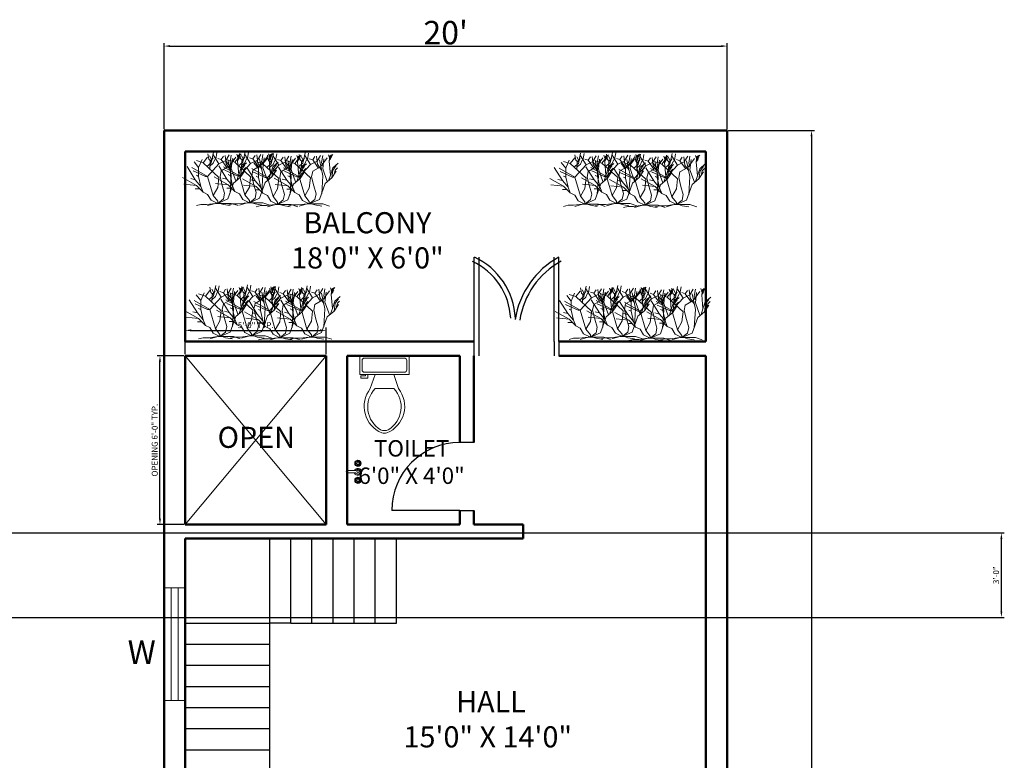
# Model space of a CAD drawing. Units: inches. Extents: x 995 to 2141, y 2161 to 2928.
# Tile 7 of 7: x 1721 to 2141, y 2613 to 2928. Entities that reach past the tile are written whole.
import ezdxf

# ---------------------------------------------------------------- set-up
doc = ezdxf.new("R2010")
doc.units = ezdxf.units.IN
for name, color, linetype, lineweight in [('A-ANNO-DIMS', 2, 'Continuous', 18), ('A-ANNO-TEXT', 7, 'Continuous', 18), ('A-AREA-IDEN', 7, 'Continuous', 25), ('A-DOOR', 3, 'Continuous', 25), ('A-FLOR-FIXT', 9, 'Continuous', 18), ('A-FLOR-OPEN', 8, 'Continuous', 13), ('A-FLOR-STRS', 7, 'Continuous', 25), ('A-GLAZ', 4, 'Continuous', 18), ('A-WALL', 7, 'Continuous', 50), ('L-PLNT-TREE', 94, 'Continuous', 13)]:
    doc.layers.add(name, color=color, linetype=linetype, lineweight=lineweight)
doc.styles.get("Standard").update_dxf_attribs({"font": 'arial.ttf'})
doc.dimstyles.new('ISO-25', dxfattribs={"dimtxt": 2.5, "dimasz": 2.5, "dimexe": 1.25, "dimexo": 0.625, "dimtad": 1, "dimdec": 0, "dimlunit": 3, "dimtxsty": 'Standard', "dimcen": 2.5, "dimadec": 0, "dimazin": 0, "dimtfac": 1, "dimtdec": 0, "dimtmove": 0, "dimatfit": 3, "dimfxl": 1, "dimarcsym": 0})

# ---------------------------------------------------------------- blocks, each defined once
blk = doc.blocks.new('*U15')
for p, q in [((-12.471, 19.775), (-12.898, 22.044)), ((-11.28, 19.619), (-12.104, 21.184)), ((-11.433, 18.289), (-10.457, 22.749)), ((-8.16, 17.76), (-10.56, 21.6)), ((-9.48, 19.775), (-8.992, 22.592)), ((-7.2, 19.68), (-6.24, 21.12)), ((-5.086, 17.741), (-5.513, 21.34)), ((-5.28, 19.2), (-3.84, 21.6)), ((-3.377, 18.602), (-2.888, 21.575)), ((-0.508, 21.888), (-0.081, 20.558)), ((-0.203, 19.149), (0.102, 21.34)), ((-0.02, 20.01), (0.896, 21.105)), ((0.041, 20.714), (1.384, 22.044)), ((0.102, 21.34), (0.835, 21.888)), ((-16.8, 16.32), (-18.72, 18.72)), ((-14.88, 18.24), (-17.76, 19.2)), ((-16.8, 16.32), (-15.36, 19.68)), ((-14.88, 18.24), (-12.96, 20.64)), ((-8.16, 12), (-14.88, 18.24)), ((-13.325, 16.724), (-11.433, 18.289)), ((-12.96, 12.48), (-8.16, 17.76)), ((-11.677, 19.071), (-12.471, 19.775)), ((-12.043, 15.628), (-11.921, 18.836)), ((-11.982, 16.802), (-10.579, 18.054)), ((-11.921, 18.836), (-10.64, 20.401)), ((-10.579, 18.054), (-9.846, 19.697)), ((-7.2, 19.68), (-8.64, 20.16)), ((-8.16, 17.76), (-5.28, 19.2)), ((-4.8, 16.32), (-7.2, 19.68)), ((-7.2, 14.88), (-3.84, 16.8)), ((-3.377, 15.315), (-5.086, 17.819)), ((-2.88, 12.96), (-4.32, 19.68)), ((-3.84, 16.8), (-0.96, 20.64)), ((-2.766, 16.802), (-3.377, 18.602)), ((-2.88, 15.84), (-2.4, 20.16)), ((0.346, 13.203), (-0.203, 19.149)), ((-0.142, 19.384), (0.59, 20.401)), ((1.323, 16.254), (3.642, 18.289)), ((1.44, 15.36), (2.88, 17.28)), ((-18.24, 11.04), (-21.755, 16.655)), ((-12.96, 12.48), (-19.68, 16.32)), ((-13.92, 12.48), (-19.2, 14.88)), ((-16.8, 12.48), (-17.76, 12.96)), ((-16.8, 12.48), (-16.8, 16.32)), ((-7.68, 12.48), (-7.2, 14.88)), ((-3.36, 5.28), (-2.88, 12.96)), ((-0.96, 10.56), (-2.88, 15.84)), ((-0.48, 10.8), (0.346, 13.203)), ((0.346, 13.203), (1.323, 16.254)), ((0.96, 12), (1.44, 15.36)), ((0.96, 12), (2.88, 14.88)), ((1.92, 13.44), (2.4, 15.36)), ((2.4, 15.36), (3.36, 16.32)), ((-17.76, 8.64), (-23.663, 11.961)), ((-17.76, 8.64), (-23.128, 9.222)), ((-18.24, 11.04), (-20.16, 11.52)), ((-15.84, 8.16), (-18.24, 11.04)), ((-14.88, 5.76), (-17.76, 8.64)), ((-15.84, 8.16), (-16.8, 12.48)), ((-12.96, 12.48), (-13.92, 12.48)), ((-10.56, 4.32), (-12.96, 12.48)), ((-8.64, 7.68), (-8.16, 12)), ((-6.72, 8.64), (-7.68, 12.48)), ((-5.76, 5.28), (-6.72, 8.64)), ((-4.32, 2.88), (-1.92, 9.6)), ((-1.92, 9.6), (0.96, 12)), ((-16.32, 7.2), (-18.24, 7.2)), ((-14.88, 5.76), (-15.84, 8.16)), ((-12.96, 4.8), (-14.88, 5.76)), ((-11.52, 2.4), (-12.96, 4.8)), ((-10.56, 4.32), (-8.64, 7.68)), ((-8.64, 1.92), (-10.56, 4.32)), ((-6.24, 2.88), (-5.76, 5.28)), ((-15.84, 0.48), (-17.76, 0)), ((-13.44, 0.48), (-15.84, 0.48)), ((-9.6, 0.96), (-13.44, 0.48)), ((-9.6, 0.96), (-12.96, 0)), ((-8.64, 0.96), (-11.52, 2.4)), ((-9.6, 0.96), (-7.68, 0.96)), ((-8.64, 0.96), (-4.32, 2.88)), ((-8.64, 0.96), (-6.24, 2.88)), ((-8.64, 0.96), (-8.64, 1.92)), ((-8.64, 0.96), (-2.88, 0.96)), ((-7.68, 0.96), (-6.24, 0.48)), ((-6.24, 0.48), (-3.36, 0)), ((-2.88, 0.96), (0, 0))]:
    blk.add_line(p, q)
blk = doc.blocks.new('Toilet - top')
for p, q in [((9.5, -6), (9.5, -2)), ((-8, -8.5), (-8, -8)), ((-7, -8), (-7, -9.5)), ((-4, -8), (-6, -14)), ((4, -8), (6, -14)), ((-10, -8.5), (-8, -8.5)), ((-10, -9.5), (-10, -8.5)), ((-7, -9.5), (-10, -9.5)), ((4, -14), (-4, -14))]:
    blk.add_line(p, q)
blk.add_lwpolyline([(10.5, -8), (10.5, 0), (-10.5, 0), (-10.5, -8)], close=True)
for points in [[(-9.5, -2), (-9.5, -6)], [(8.5, -1), (-8.5, -1)], [(-8.5, -7), (8.5, -7)]]:
    blk.add_lwpolyline(points)
for centre, radius, start, end in [((-8.62, -1.88), 0.884, 81.8699, 188.1301), ((8.62, -1.88), 0.884, 351.8699, 98.1301), ((-8.62, -6.12), 0.884, 171.8699, 278.1301), ((8.62, -6.12), 0.884, 261.8699, 8.1301), ((3.52, -21.58), 12.17, 141.4691, 247.9714), ((4.2, -21.82), 11.33, 136.3677, 238.9468), ((-3.52, -21.58), 12.17, 292.0284, 38.5307), ((-4.2, -21.82), 11.33, 301.053, 43.6321), ((0, -27.88), 4, 245.7318, 294.2682), ((0, -29), 4, 254.8605, 285.1395)]:
    blk.add_arc(centre, radius, start, end)
blk = doc.blocks.new('Faucet - Bathroom top')
for p, q in [((-4.107, 0.125), (-4.375, 0.125)), ((-3.75, 0.4788), (-3.75, 0.75)), ((-3.5, 0.482), (-3.5, 0.75)), ((-3.1461, 0.125), (-2.875, 0.125)), ((3.143, 0.125), (2.875, 0.125)), ((3.5, 0.4788), (3.5, 0.75)), ((3.75, 0.482), (3.75, 0.75)), ((4.1039, 0.125), (4.375, 0.125)), ((-4.1039, -0.125), (-4.375, -0.125)), ((-3.75, -0.4821), (-3.75, -0.75)), ((-3.5, -0.4789), (-3.5, -0.75)), ((-3.143, -0.125), (-2.875, -0.125)), ((-0.5, -0.8639), (-0.5, -4.5)), ((0.5, -4.5), (0.5, -0.8631)), ((3.1461, -0.125), (2.875, -0.125)), ((3.5, -0.4821), (3.5, -0.75)), ((3.75, -0.4789), (3.75, -0.75)), ((4.107, -0.125), (4.375, -0.125))]:
    blk.add_line(p, q)
for centre, radius in [((-3.625, 0), 1.375), ((-4.625, 0), 0.2795), ((-3.625, 0), 0.5), ((-3.625, 1), 0.2795), ((-2.625, 0), 0.2795), ((0, 0), 0.5), ((3.625, 0), 1.375), ((2.625, 0), 0.2795), ((3.625, 0), 0.5), ((3.625, 1), 0.2795), ((4.625, 0), 0.2795), ((-3.625, -1), 0.2795), ((3.625, -1), 0.2795)]:
    blk.add_circle(centre, radius)
for centre, radius, start, end in [((-3.625, 0), 1, 105.2407, 164.2093), ((-3.625, 0), 1, 16.44125, 74.07887), ((0, 0), 1.5, 289.6514, 250.3603), ((0, 0), 1, 300.3431, 239.7554), ((3.625, 0), 1, 106.12, 164.0884), ((3.625, 0), 1, 16.23422, 73.90469), ((-3.625, 0), 1, 196.2342, 253.9047), ((-3.625, 0), 1, 286.12, 344.0884), ((3.625, 0), 1, 196.4413, 254.0789), ((3.625, 0), 1, 285.2407, 344.2093), ((0, -4.5), 0.5, 180, 0)]:
    blk.add_arc(centre, radius, start, end)
blk = doc.blocks.new('*D19')
at = {"layer": 'A-ANNO-DIMS', "color": 0, "lineweight": -2, "transparency": 16777216}
for p, q in [((1783.1, 2881.73), (1783.1, 2918.35)), ((2023.1, 2881.73), (2023.1, 2918.35)), ((1785.6, 2917.1), (2020.6, 2917.1))]:
    blk.add_line(p, q, dxfattribs=at)
at = {"layer": 'A-ANNO-DIMS', "color": 0, "transparency": 16777216}
for points in [[(1785.6, 2917.52), (1785.6, 2916.68), (1783.1, 2917.1)], [(2020.6, 2917.52), (2020.6, 2916.68), (2023.1, 2917.1)]]:
    blk.add_solid(points, dxfattribs=at)
at = {"layer": 'Defpoints', "color": 0, "transparency": 16777216}
for p in [(2023.1, 2917.1), (1783.1, 2881.1), (2023.1, 2881.1)]:
    blk.add_point(p, dxfattribs=at)
at = {"layer": 'A-ANNO-DIMS', "color": 0, "transparency": 16777216, "insert": (1903.1, 2922.83), "char_height": 2.5, "attachment_point": 5}
blk.add_mtext("{\\H4x;20'}", dxfattribs=at)
blk = doc.blocks.new('*D20')
at = {"layer": 'A-ANNO-DIMS', "color": 0, "lineweight": -2, "transparency": 16777216}
for p, q in [((2023.72, 2881.1), (2060.35, 2881.1)), ((2059.1, 2878.6), (2059.1, 2283.6)), ((2023.72, 2281.1), (2060.35, 2281.1))]:
    blk.add_line(p, q, dxfattribs=at)
at = {"layer": 'A-ANNO-DIMS', "color": 0, "transparency": 16777216}
for points in [[(2058.68, 2878.6), (2059.51, 2878.6), (2059.1, 2881.1)], [(2058.68, 2283.6), (2059.51, 2283.6), (2059.1, 2281.1)]]:
    blk.add_solid(points, dxfattribs=at)
at = {"layer": 'Defpoints', "color": 0, "transparency": 16777216}
for p in [(2023.1, 2881.1), (2023.1, 2281.1), (2059.1, 2281.1)]:
    blk.add_point(p, dxfattribs=at)
at = {"layer": 'A-ANNO-DIMS', "color": 0, "transparency": 16777216, "insert": (2053.37, 2581.1), "char_height": 2.5, "attachment_point": 5, "rotation": 90}
blk.add_mtext("{\\H4x;50'}", dxfattribs=at)
blk = doc.blocks.new('WIN-48IN')
for p, q in [((0, 48), (0, 0)), ((9, 48), (0, 48)), ((3, 48), (3, 0)), ((6, 0), (6, 48)), ((9, 0), (9, 48)), ((0, 0), (9, 0))]:
    blk.add_line(p, q)
blk = doc.blocks.new('OPENING-CROSS-60X72')
for p, q in [((60, 72), (0, 0)), ((0, 72), (60, 0))]:
    blk.add_line(p, q)
blk = doc.blocks.new('*D38')
at = {"layer": 'A-ANNO-DIMS', "color": 0, "lineweight": -2, "transparency": 16777216}
for p, q in [((1791.47, 2785.1), (1780.05, 2785.1)), ((1781.3, 2715.6), (1781.3, 2782.6)), ((1791.47, 2713.1), (1780.05, 2713.1))]:
    blk.add_line(p, q, dxfattribs=at)
at = {"layer": 'A-ANNO-DIMS', "color": 0, "transparency": 16777216}
for points in [[(1780.88, 2782.6), (1781.71, 2782.6), (1781.3, 2785.1)], [(1780.88, 2715.6), (1781.71, 2715.6), (1781.3, 2713.1)]]:
    blk.add_solid(points, dxfattribs=at)
at = {"layer": 'Defpoints', "color": 0, "transparency": 16777216}
for p in [(1781.3, 2785.1), (1792.1, 2785.1), (1792.1, 2713.1)]:
    blk.add_point(p, dxfattribs=at)
at = {"layer": 'A-ANNO-DIMS', "color": 0, "transparency": 16777216, "insert": (1779.38, 2749.1), "char_height": 2.5, "attachment_point": 5, "rotation": 90}
blk.add_mtext('OPENING 6\'-0" TYP.', dxfattribs=at)
blk = doc.blocks.new('*D39')
at = {"layer": 'A-ANNO-DIMS', "color": 0, "lineweight": -2, "transparency": 16777216}
for p, q in [((1792.1, 2785.73), (1792.1, 2797.15)), ((1852.1, 2785.73), (1852.1, 2797.15)), ((1794.6, 2795.9), (1849.6, 2795.9))]:
    blk.add_line(p, q, dxfattribs=at)
at = {"layer": 'A-ANNO-DIMS', "color": 0, "transparency": 16777216}
for points in [[(1794.6, 2796.32), (1794.6, 2795.48), (1792.1, 2795.9)], [(1849.6, 2796.32), (1849.6, 2795.48), (1852.1, 2795.9)]]:
    blk.add_solid(points, dxfattribs=at)
at = {"layer": 'Defpoints', "color": 0, "transparency": 16777216}
for p in [(1852.1, 2795.9), (1792.1, 2785.1), (1852.1, 2785.1)]:
    blk.add_point(p, dxfattribs=at)
at = {"layer": 'A-ANNO-DIMS', "color": 0, "transparency": 16777216, "insert": (1822.1, 2797.8), "char_height": 2.5, "attachment_point": 5}
blk.add_mtext('5\'-0" TYP.', dxfattribs=at)
blk = doc.blocks.new('*D64')
at = {"layer": 'A-ANNO-DIMS', "color": 0, "lineweight": -2, "transparency": 16777216}
for p, q in [((1532.63, 2709.52), (2141.3, 2709.52)), ((2140.05, 2676.02), (2140.05, 2707.02)), ((1532.63, 2673.52), (2141.3, 2673.52))]:
    blk.add_line(p, q, dxfattribs=at)
at = {"layer": 'A-ANNO-DIMS', "color": 0, "transparency": 16777216}
for points in [[(2139.63, 2707.02), (2140.46, 2707.02), (2140.05, 2709.52)], [(2139.63, 2676.02), (2140.46, 2676.02), (2140.05, 2673.52)]]:
    blk.add_solid(points, dxfattribs=at)
at = {"layer": 'Defpoints', "color": 0, "transparency": 16777216}
for p in [(1532, 2709.52), (2140.05, 2709.52), (1532, 2673.52)]:
    blk.add_point(p, dxfattribs=at)
at = {"layer": 'A-ANNO-DIMS', "color": 0, "transparency": 16777216, "insert": (2138.14, 2691.52), "char_height": 2.5, "attachment_point": 5, "rotation": 90}
blk.add_mtext('3\'-0"', dxfattribs=at)

msp = doc.modelspace()

# ---------------------------------------------------------------- linework, layer by layer
at = {"layer": 'A-DOOR'}
for p, q in [((1915.33, 2791.1), (1915.33, 2827.1)), ((1917.33, 2791.1), (1917.33, 2827.1)), ((1949.33, 2791.1), (1949.33, 2827.1)), ((1951.33, 2791.1), (1951.33, 2827.1)), ((1915.33, 2785.1), (1915.33, 2791.1)), ((1917.33, 2785.1), (1917.33, 2791.1)), ((1949.33, 2791.1), (1949.33, 2785.1)), ((1951.33, 2791.1), (1951.33, 2785.1)), ((1915.1, 2748.1), (1909.1, 2748.1)), ((1909.1, 2719.1), (1880.1, 2719.1)), ((1909.1, 2719.1), (1915.1, 2719.1))]:
    msp.add_line(p, q, dxfattribs=at)
for centre, radius, start, end in [((1902.65, 2799.67), 30.22, 2.781, 65.1814), ((1969.03, 2794.92), 36.73, 118.8094, 171.2426), ((1969.03, 2794.92), 34.73, 118.8094, 171.2426), ((1902.65, 2799.67), 28.22, 2.781, 65.1814), ((1909.1, 2719.1), 29, 90, 180)]:
    msp.add_arc(centre, radius, start, end, dxfattribs=at)
at = {"layer": 'A-FLOR-STRS'}
for p, q in [((1828.1, 2539.1), (1828.1, 2707.1)), ((1837.1, 2671.1), (1837.1, 2707.1)), ((1846.1, 2671.1), (1846.1, 2707.1)), ((1855.1, 2671.1), (1855.1, 2707.1)), ((1864.1, 2671.1), (1864.1, 2707.1)), ((1873.1, 2671.1), (1873.1, 2707.1)), ((1882.1, 2671.1), (1882.1, 2707.1)), ((1792.1, 2671.1), (1828.1, 2671.1)), ((1837.1, 2671.1), (1828.1, 2671.1)), ((1837.1, 2671.1), (1882.1, 2671.1)), ((1792.1, 2662.1), (1828.1, 2662.1)), ((1792.1, 2653.1), (1828.1, 2653.1)), ((1792.1, 2644.1), (1828.1, 2644.1)), ((1792.1, 2635.1), (1828.1, 2635.1)), ((1792.1, 2626.1), (1828.1, 2626.1)), ((1792.1, 2617.1), (1828.1, 2617.1))]:
    msp.add_line(p, q, dxfattribs=at)
at = {"layer": 'A-WALL'}
for p, q in [((1783.1, 2881.1), (2023.1, 2881.1)), ((1783.1, 2281.1), (1783.1, 2881.1)), ((2023.1, 2881.1), (2023.1, 2281.1)), ((1792.1, 2872.1), (2014.1, 2872.1)), ((1792.1, 2791.1), (1792.1, 2872.1)), ((2014.1, 2872.1), (2014.1, 2791.1)), ((1792.1, 2791.1), (1915.33, 2791.1)), ((1951.33, 2791.1), (2014.1, 2791.1)), ((1792.1, 2785.1), (1852.1, 2785.1)), ((1792.1, 2713.1), (1792.1, 2785.1)), ((1792.1, 2713.1), (1792.1, 2785.1)), ((1852.1, 2713.1), (1852.1, 2785.1)), ((1861.1, 2785.1), (1909.1, 2785.1)), ((1861.1, 2713.1), (1861.1, 2785.1)), ((1909.1, 2748.1), (1909.1, 2785.1)), ((1915.1, 2785.1), (1915.33, 2785.1)), ((1915.1, 2748.1), (1915.1, 2785.1)), ((1951.33, 2785.1), (2014.1, 2785.1)), ((2014.1, 2785.1), (2014.1, 2713.1)), ((1909.1, 2713.1), (1909.1, 2719.1)), ((1909.1, 2713.1), (1909.1, 2719.1)), ((1915.1, 2713.1), (1915.1, 2719.1)), ((1792.1, 2713.1), (1852.1, 2713.1)), ((1861.1, 2713.1), (1909.1, 2713.1)), ((1915.1, 2713.1), (1936.1, 2713.1)), ((1936.1, 2713.1), (1936.1, 2707.1)), ((2014.1, 2713.1), (2014.1, 2699.43)), ((1792.1, 2707.1), (1936.1, 2707.1)), ((1792.1, 2539.1), (1792.1, 2707.1)), ((2014.1, 2707.1), (2014.1, 2539.1))]:
    msp.add_line(p, q, dxfattribs=at)

# ---------------------------------------------------------------- block references
at = {"layer": 'A-FLOR-FIXT'}
msp.add_blockref('Toilet - top', (1876.99, 2785.06), dxfattribs=at)
at = {"layer": 'A-FLOR-FIXT', "rotation": 270}
msp.add_blockref('Faucet - Bathroom top', (1865.7, 2735.59), dxfattribs=at)
at = {"layer": 'A-FLOR-OPEN'}
msp.add_blockref('OPENING-CROSS-60X72', (1792.1, 2713.1), dxfattribs=at)
at = {"layer": 'A-GLAZ'}
msp.add_blockref('WIN-48IN', (1783.1, 2638.1), dxfattribs=at)
at = {"layer": 'L-PLNT-TREE'}
for p in [(1814.59, 2849.07), (1828.1, 2849.33), (1853.61, 2848.87), (1971.12, 2848.75), (1984.63, 2849.01), (1840.1, 2848.61), (1996.63, 2848.29), (2010.14, 2848.55), (1815.52, 2792.28), (1829.03, 2792.54), (1841.03, 2791.82), (1854.54, 2792.08), (1973.46, 2792.03), (1986.97, 2792.29), (1998.97, 2791.57), (2012.48, 2791.83)]:
    msp.add_blockref('*U15', p, dxfattribs=at)

# ---------------------------------------------------------------- texts
at = {"layer": 'A-ANNO-TEXT', "insert": (1767.52, 2663.71), "char_height": 10, "attachment_point": 1}
msp.add_mtext_dynamic_manual_height_columns('W', width=112.484, gutter_width=12.5, heights=[0], dxfattribs=at)
at = {"layer": 'A-AREA-IDEN', "attachment_point": 1}
for s, width, insert, char_height in [('\\pxqc;BALCONY \\P18\'0" X 6\'0"', 118.2971, (1810.6, 2846.29), 9), ('\\pxqc;OPEN ', 52.2467, (1796.26, 2754.81), 9), ('\\pxqc;TOILET\\P6\'0" X 4\'0"', 53.0246, (1862.07, 2749.1), 7), ('\\pxqc; HALL \\P15\'0" X 14\'0"', 103.3264, (1869.4, 2642.11), 9)]:
    msp.add_mtext_dynamic_manual_height_columns(s, width=width, gutter_width=12.5, heights=[0], dxfattribs=dict(at, insert=insert, char_height=char_height))

# ---------------------------------------------------------------- dimensions: what is measured, and where the dimension line sits
at = {"layer": 'A-ANNO-DIMS'}
for base, p1, p2, text, override, picture, middle in [((2023.1, 2917.1), (1783.1, 2881.1), (2023.1, 2881.1), "{\\H4x;20'}", {"dimclrd": 0, "dimclre": 0, "dimclrt": 0}, '*D19', (1903.1, 2922.83)), ((1852.1, 2795.9), (1792.1, 2785.1), (1852.1, 2785.1), '<> TYP.', {"dimdec": 1, "dimlfac": 1, "dimrnd": 0, "dimzin": 1, "dimdsep": 46, "dimlunit": 4, "dimfrac": 2}, '*D39', (1822.1, 2797.8))]:
    dim = msp.add_linear_dim(base=base, p1=p1, p2=p2, text=text, dimstyle='ISO-25', override=override, dxfattribs=at)
    dim.commit()
    dim.dimension.update_dxf_attribs({"geometry": picture, "text_midpoint": middle})
for base, p1, p2, text, override, picture, middle in [((2059.1, 2281.1), (2023.1, 2881.1), (2023.1, 2281.1), "{\\H4x;50'}", {"dimclrd": 0, "dimclre": 0, "dimclrt": 0}, '*D20', (2053.37, 2581.1)), ((1781.3, 2785.1), (1792.1, 2713.1), (1792.1, 2785.1), 'OPENING <> TYP.', {"dimdec": 1, "dimlfac": 1, "dimrnd": 0, "dimzin": 1, "dimdsep": 46, "dimlunit": 4, "dimfrac": 2}, '*D38', (1779.38, 2749.1))]:
    dim = msp.add_linear_dim(base=base, p1=p1, p2=p2, angle=90, text=text, dimstyle='ISO-25', override=override, dxfattribs=at)
    dim.commit()
    dim.dimension.update_dxf_attribs({"geometry": picture, "text_midpoint": middle})
dim = msp.add_linear_dim(base=(2140.05, 2709.52), p1=(1532, 2673.52), p2=(1532, 2709.52), angle=90, dimstyle='ISO-25', override={"dimdec": 1, "dimlfac": 1, "dimrnd": 0, "dimzin": 1, "dimdsep": 46, "dimlunit": 4, "dimfrac": 2}, dxfattribs=at)
dim.commit()
dim.dimension.update_dxf_attribs({"geometry": '*D64', "text_midpoint": (2138.14, 2691.52)})

doc.saveas('drawing.dxf')
